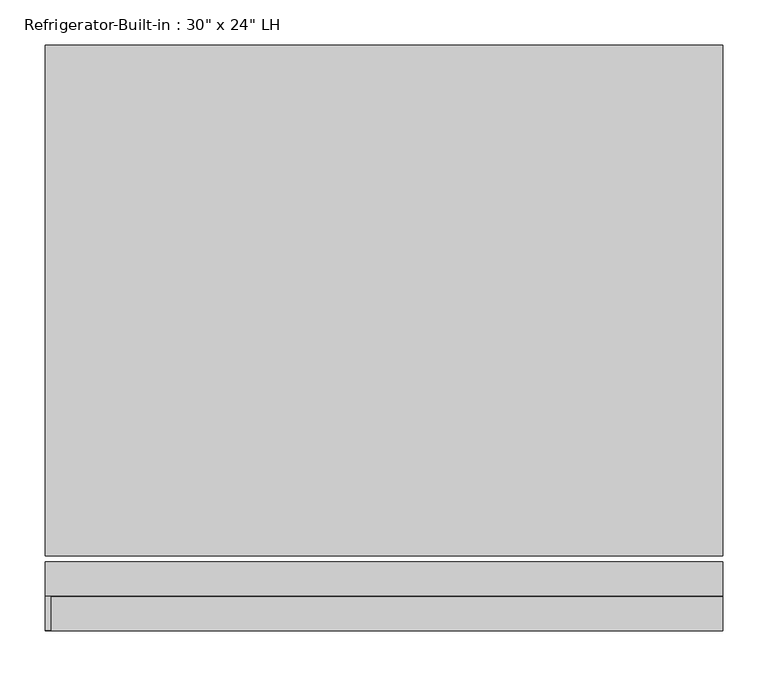
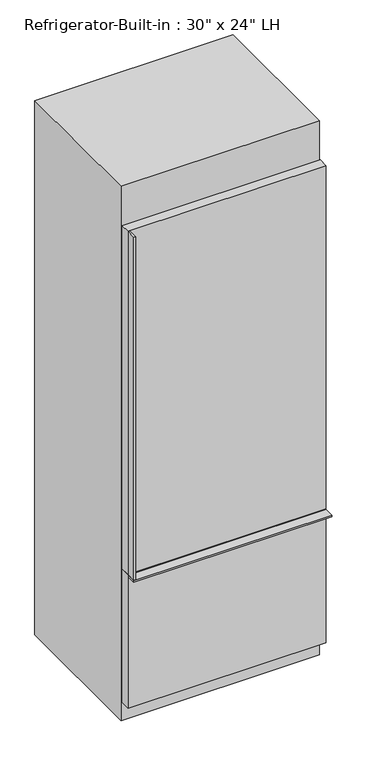
"""IFC4 building model written with IfcOpenShell, lengths in millimetres: proxy geometry."""

from ifc_helpers import new_model, si_unit, frame, origin, origin_with_axes, place, context, project, spatial, polyline, outline, extrude, source, transform, mapped, element, save


def proxy_19935bb1(model_context):
    return source(origin(), model_context, "Body", "SweptSolid", [
        extrude(outline(polyline([(374.65, 290.1239715), (374.65, -275.0260285), (-374.65, -275.0260285), (-374.65, 290.1239715), (374.65, 290.1239715)])), origin_with_axes(), (0.0, 0.0, 1.0), 2133.6),
        extrude(outline(polyline([(374.65, -281.3760285), (374.65, -319.4760285), (-374.65, -319.4760285), (-374.65, -281.3760285), (374.65, -281.3760285)])), frame((0.0, 0.0, 611.1875), z_axis=(0.0, 0.0, 1.0), x_axis=(1.0, 0.0, 0.0)), (0.0, 0.0, 1.0), 1370.0125),
        extrude(outline(polyline([(374.65, -281.3760285), (374.65, -319.4760285), (-374.65, -319.4760285), (-374.65, -281.3760285), (374.65, -281.3760285)])), frame((0.0, 0.0, 76.2), z_axis=(0.0, 0.0, 1.0), x_axis=(1.0, 0.0, 0.0)), (0.0, 0.0, 1.0), 531.8125),
        extrude(outline(polyline([(374.65, -319.4760285), (374.65, -357.5760285), (-374.65, -357.5760285), (-374.65, -319.4760285), (374.65, -319.4760285)])), frame((0.0, 0.0, 601.6625), z_axis=(0.0, 0.0, 1.0), x_axis=(1.0, 0.0, 0.0)), (0.0, 0.0, 1.0), 6.35),
        extrude(outline(polyline([(-374.65, -319.4760285), (-368.3, -319.4760285), (-368.3, -357.5760285), (-374.65, -357.5760285), (-374.65, -319.4760285)])), frame((0.0, 0.0, 611.1875), z_axis=(0.0, 0.0, 1.0), x_axis=(1.0, 0.0, 0.0)), (0.0, 0.0, 1.0), 1370.0125),
    ])


if __name__ == "__main__":
    model = new_model("IFC4")
    model_context = context("Model", 3, world=origin())
    ifc_project = project(units=[si_unit("LENGTHUNIT", "METRE", prefix="MILLI")], contexts=[model_context])
    site = spatial("IfcSite", under=ifc_project)
    building = spatial("IfcBuilding", under=site)
    placement = place(None, origin())
    proxy_shape = proxy_19935bb1(model_context)
    element("IfcBuildingElementProxy", 1, Name="Refrigerator-Built-in : 30\" x 24\" LH", ObjectType="Refrigerator-Built-in : 30\" x 24\" LH", at=placement, inside=building, context=model_context, shape_type="MappedRepresentation", body=[
        mapped(proxy_shape, transform((0.0, 0.0, 0.0), x_axis=(1.0, 0.0, 0.0), y_axis=(0.0, 1.0, 0.0), z_axis=(0.0, 0.0, 1.0))),
    ])
    save(model, "model.ifc")

# Revit data of these elements
# Type "Refrigerator-Built-in : 30\" x 24\" LH"
#   Assembly Code = "E1090400"
#   Depth = 2' - 0"
#   Handle = 0' - 0 1/4"
#   Height = 7' - 0"
#   Top Door Height = 5' - 0"
#   Width = 2' - 5 1/2"
#   Material = Metal - Paint Finish - Ivory,Glossy
#   Default Elevation = 0
# Element 1 (IfcBuildingElementProxy, "Refrigerator-Built-in : 30\" x 24\" LH")
#   Materials on its faces: "Metal - Paint Finish - Ivory,Glossy", "Metal - Chrome"
# Materials
#   "Metal - Paint Finish - Ivory,Glossy": colour RGB 247 247 239, transparency 0
#   "Metal - Chrome": colour RGB 17 17 17, transparency 0
